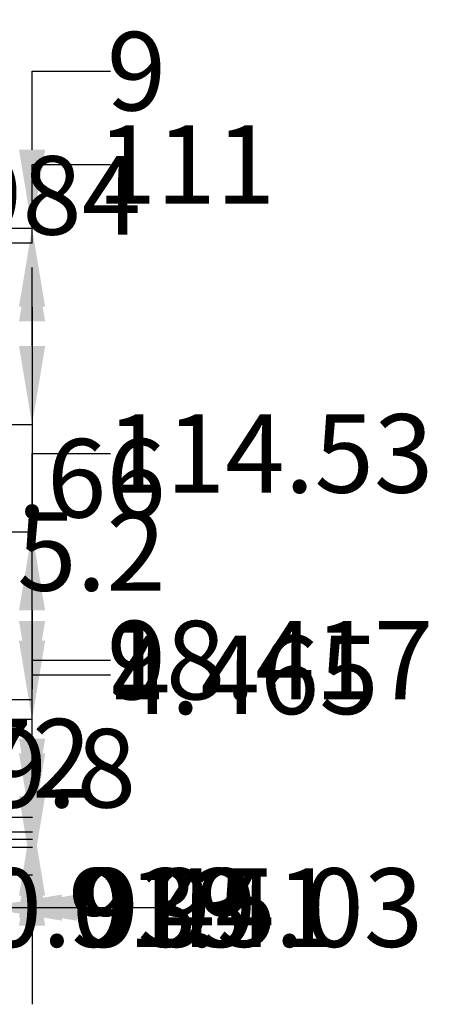
# Model space of a CAD drawing. Units: inches. Extents: x 131 to 858, y -65 to 554.
# Tile 4 of 4: x 605 to 858, y -48 to 554. Entities that reach past the tile are written whole.
import ezdxf

# ---------------------------------------------------------------- set-up
doc = ezdxf.new("R2010")
doc.units = ezdxf.units.IN
doc.header["$MEASUREMENT"] = 0
doc.layers.add('A-ANNO-DIMS', color=2, linetype='Continuous', lineweight=18)
doc.styles.get("Standard").update_dxf_attribs({"font": 'arial.ttf'})
doc.dimstyles.get("Standard").update_dxf_attribs({"dimtxt": 48, "dimasz": 48, "dimexe": 0.18, "dimexo": 0.0625, "dimgap": 0.09, "dimtad": 0, "dimtih": 1, "dimtoh": 1, "dimdec": 0, "dimrnd": 72, "dimzin": 0, "dimdsep": 46, "dimlunit": 3, "dimtxsty": 'Standard', "dimcen": 0.09, "dimadec": 0, "dimazin": 0, "dimtfac": 1, "dimtdec": 0, "dimtofl": 0, "dimtmove": 0, "dimatfit": 3, "dimfxl": 1, "dimtolj": 1, "dimtzin": 0, "dimarcsym": 0})

# ---------------------------------------------------------------- blocks, each defined once
blk = doc.blocks.new('*D5')
at = {"layer": 'A-ANNO-DIMS', "color": 0, "lineweight": -2, "transparency": 16777216}
for p, q in [((325.03, 446.65), (277.03, 446.65)), ((373.03, 426.61), (373.03, 446.83)), ((386.01, 421.76), (386.01, 446.83)), ((434.01, 446.65), (482.01, 446.65))]:
    blk.add_line(p, q, dxfattribs=at)
at = {"layer": 'A-ANNO-DIMS', "color": 0, "transparency": 16777216}
for points in [[(325.03, 454.65), (325.03, 438.65), (373.03, 446.65)], [(434.01, 454.65), (434.01, 438.65), (386.01, 446.65)]]:
    blk.add_solid(points, dxfattribs=at)
at = {"layer": 'Defpoints', "color": 0, "transparency": 16777216}
for p in [(386.01, 446.65), (373.03, 426.55), (386.01, 421.7)]:
    blk.add_point(p, dxfattribs=at)
at = {"layer": 'A-ANNO-DIMS', "color": 0, "transparency": 16777216, "insert": (579.38, 446.65), "char_height": 48, "attachment_point": 5}
blk.add_mtext('\\A1;12.984', dxfattribs=at)
blk = doc.blocks.new('*D11')
at = {"layer": 'A-ANNO-DIMS', "color": 0, "lineweight": -2, "transparency": 16777216}
for p, q in [((395.014446, 31.273524), (395.014446, 11.056024)), ((539.014446, 31.273524), (539.014446, 11.056024)), ((347.014446, 11.236024), (299.014446, 11.236024)), ((587.014446, 11.236024), (635.014446, 11.236024))]:
    blk.add_line(p, q, dxfattribs=at)
at = {"layer": 'A-ANNO-DIMS', "color": 0, "transparency": 16777216}
for points in [[(347.014446, 19.236024), (347.014446, 3.236024), (395.014446, 11.236024)], [(587.014446, 19.236024), (587.014446, 3.236024), (539.014446, 11.236024)]]:
    blk.add_solid(points, dxfattribs=at)
at = {"layer": 'Defpoints', "color": 0, "transparency": 16777216}
for p in [(395.014446, 31.336024), (539.014446, 31.336024), (539.014446, 11.236024)]:
    blk.add_point(p, dxfattribs=at)
at = {"layer": 'A-ANNO-DIMS', "color": 0, "transparency": 16777216, "insert": (467.014446, 11.236024), "char_height": 48, "attachment_point": 5}
blk.add_mtext('\\A1;144', dxfattribs=at)
blk = doc.blocks.new('*D12')
at = {"layer": 'A-ANNO-DIMS', "color": 0, "lineweight": -2, "transparency": 16777216}
for p, q in [((539.01, 31.27), (539.01, 11.06)), ((548.01, 31.27), (548.01, 11.06)), ((491.01, 11.24), (443.01, 11.24)), ((596.01, 11.24), (644.01, 11.24))]:
    blk.add_line(p, q, dxfattribs=at)
at = {"layer": 'A-ANNO-DIMS', "color": 0, "transparency": 16777216}
for points in [[(491.01, 19.24), (491.01, 3.24), (539.01, 11.24)], [(596.01, 19.24), (596.01, 3.24), (548.01, 11.24)]]:
    blk.add_solid(points, dxfattribs=at)
at = {"layer": 'Defpoints', "color": 0, "transparency": 16777216}
for p in [(539.01, 31.34), (548.01, 31.34), (548.01, 11.24)]:
    blk.add_point(p, dxfattribs=at)
at = {"layer": 'A-ANNO-DIMS', "color": 0, "transparency": 16777216, "insert": (659.89, 11.24), "char_height": 48, "attachment_point": 5}
blk.add_mtext('\\A1;9', dxfattribs=at)
blk = doc.blocks.new('*D13')
at = {"layer": 'A-ANNO-DIMS', "color": 0, "lineweight": -2, "transparency": 16777216}
for p, q in [((592.04, 126.29), (592.04, 11.06)), ((548.01, 31.27), (548.01, 11.06)), ((500.01, 11.24), (452.01, 11.24)), ((640.04, 11.24), (688.04, 11.24))]:
    blk.add_line(p, q, dxfattribs=at)
at = {"layer": 'A-ANNO-DIMS', "color": 0, "transparency": 16777216}
for points in [[(500.01, 19.24), (500.01, 3.24), (548.01, 11.24)], [(640.04, 19.24), (640.04, 3.24), (592.04, 11.24)]]:
    blk.add_solid(points, dxfattribs=at)
at = {"layer": 'Defpoints', "color": 0, "transparency": 16777216}
for p in [(592.04, 126.36), (548.01, 31.34), (592.04, 11.24)]:
    blk.add_point(p, dxfattribs=at)
at = {"layer": 'A-ANNO-DIMS', "color": 0, "transparency": 16777216, "insert": (770.09, 11.24), "char_height": 48, "attachment_point": 5}
blk.add_mtext('\\A1;44.03', dxfattribs=at)
blk = doc.blocks.new('*D14')
at = {"layer": 'A-ANNO-DIMS', "color": 0, "lineweight": -2, "transparency": 16777216}
for p, q in [((592.11, 426.55), (612.82, 426.55)), ((612.64, 378.55), (612.64, 253.56)), ((612.64, 79.34), (612.64, 204.33)), ((233.08, 31.34), (612.82, 31.34))]:
    blk.add_line(p, q, dxfattribs=at)
at = {"layer": 'A-ANNO-DIMS', "color": 0, "transparency": 16777216}
for points in [[(604.64, 378.55), (620.64, 378.55), (612.64, 426.55)], [(604.64, 79.34), (620.64, 79.34), (612.64, 31.34)]]:
    blk.add_solid(points, dxfattribs=at)
at = {"layer": 'Defpoints', "color": 0, "transparency": 16777216}
for p in [(592.04, 426.55), (612.64, 426.55), (233.01, 31.34)]:
    blk.add_point(p, dxfattribs=at)
at = {"layer": 'A-ANNO-DIMS', "color": 0, "transparency": 16777216, "insert": (612.64, 228.94), "char_height": 48, "attachment_point": 5}
blk.add_mtext('\\A1;395.2', dxfattribs=at)
blk = doc.blocks.new('*D19')
at = {"layer": 'A-ANNO-DIMS', "color": 0, "lineweight": -2, "transparency": 16777216}
for p, q in [((612.64, 105.55), (612.64, 153.55)), ((612.64, 153.55), (660.64, 153.55)), ((242.08, 57.55), (612.82, 57.55)), ((242.08, 53.09), (612.82, 53.09)), ((612.64, 5.09), (612.64, -42.91))]:
    blk.add_line(p, q, dxfattribs=at)
at = {"layer": 'A-ANNO-DIMS', "color": 0, "transparency": 16777216}
for points in [[(604.64, 105.55), (620.64, 105.55), (612.64, 57.55)], [(604.64, 5.09), (620.64, 5.09), (612.64, 53.09)]]:
    blk.add_solid(points, dxfattribs=at)
at = {"layer": 'Defpoints', "color": 0, "transparency": 16777216}
for p in [(242.01, 57.55), (612.64, 57.55), (242.01, 53.09)]:
    blk.add_point(p, dxfattribs=at)
at = {"layer": 'A-ANNO-DIMS', "color": 0, "transparency": 16777216, "insert": (742.86, 153.55), "char_height": 48, "attachment_point": 5}
blk.add_mtext('\\A1;4.465', dxfattribs=at)
blk = doc.blocks.new('*D20')
at = {"layer": 'A-ANNO-DIMS', "color": 0, "lineweight": -2, "transparency": 16777216}
for p, q in [((612.64, 114.55), (612.64, 162.55)), ((612.64, 162.55), (660.64, 162.55)), ((242.08, 66.55), (612.82, 66.55)), ((242.08, 57.55), (612.82, 57.55)), ((612.64, 9.55), (612.64, -38.45))]:
    blk.add_line(p, q, dxfattribs=at)
at = {"layer": 'A-ANNO-DIMS', "color": 0, "transparency": 16777216}
for points in [[(604.64, 114.55), (620.64, 114.55), (612.64, 66.55)], [(604.64, 9.55), (620.64, 9.55), (612.64, 57.55)]]:
    blk.add_solid(points, dxfattribs=at)
at = {"layer": 'Defpoints', "color": 0, "transparency": 16777216}
for p in [(242.01, 66.55), (612.64, 66.55), (242.01, 57.55)]:
    blk.add_point(p, dxfattribs=at)
at = {"layer": 'A-ANNO-DIMS', "color": 0, "transparency": 16777216, "insert": (676.51, 162.55), "char_height": 48, "attachment_point": 5}
blk.add_mtext('\\A1;9', dxfattribs=at)
blk = doc.blocks.new('*D22')
at = {"layer": 'A-ANNO-DIMS', "color": 0, "lineweight": -2, "transparency": 16777216}
for p, q in [((612.64, 114.55), (612.64, 162.55)), ((612.64, 162.55), (660.64, 162.55)), ((395.08, 66.55), (612.82, 66.55)), ((395.08, 48.13), (612.82, 48.13)), ((612.64, 0.13), (612.64, -47.87))]:
    blk.add_line(p, q, dxfattribs=at)
at = {"layer": 'A-ANNO-DIMS', "color": 0, "transparency": 16777216}
for points in [[(604.64, 114.55), (620.64, 114.55), (612.64, 66.55)], [(604.64, 0.13), (620.64, 0.13), (612.64, 48.13)]]:
    blk.add_solid(points, dxfattribs=at)
at = {"layer": 'Defpoints', "color": 0, "transparency": 16777216}
for p in [(395.01, 66.55), (612.64, 66.55), (395.01, 48.13)]:
    blk.add_point(p, dxfattribs=at)
at = {"layer": 'A-ANNO-DIMS', "color": 0, "transparency": 16777216, "insert": (758.11, 162.55), "char_height": 48, "attachment_point": 5}
blk.add_mtext('\\A1;18.417', dxfattribs=at)
blk = doc.blocks.new('*D30')
at = {"layer": 'A-ANNO-DIMS', "color": 0, "lineweight": -2, "transparency": 16777216}
for p, q in [((612.64, 417.55), (612.64, 465.55)), ((612.64, 465.55), (660.64, 465.55)), ((592.11, 417.55), (612.82, 417.55)), ((612.64, 354.55), (612.64, 369.55)), ((443.08, 306.55), (612.82, 306.55))]:
    blk.add_line(p, q, dxfattribs=at)
at = {"layer": 'A-ANNO-DIMS', "color": 0, "transparency": 16777216}
for points in [[(604.64, 369.55), (620.64, 369.55), (612.64, 417.55)], [(604.64, 354.55), (620.64, 354.55), (612.64, 306.55)]]:
    blk.add_solid(points, dxfattribs=at)
at = {"layer": 'Defpoints', "color": 0, "transparency": 16777216}
for p in [(592.04, 417.55), (612.64, 417.55), (443.01, 306.55)]:
    blk.add_point(p, dxfattribs=at)
at = {"layer": 'A-ANNO-DIMS', "color": 0, "transparency": 16777216, "insert": (706.86, 465.55), "char_height": 48, "attachment_point": 5}
blk.add_mtext('\\A1;111', dxfattribs=at)
blk = doc.blocks.new('*D31')
at = {"layer": 'A-ANNO-DIMS', "color": 0, "lineweight": -2, "transparency": 16777216}
for p, q in [((612.64, 474.55), (612.64, 522.55)), ((612.64, 522.55), (660.64, 522.55)), ((592.11, 426.55), (612.82, 426.55)), ((592.11, 417.55), (612.82, 417.55)), ((612.64, 369.55), (612.64, 321.55))]:
    blk.add_line(p, q, dxfattribs=at)
at = {"layer": 'A-ANNO-DIMS', "color": 0, "transparency": 16777216}
for points in [[(604.64, 474.55), (620.64, 474.55), (612.64, 426.55)], [(604.64, 369.55), (620.64, 369.55), (612.64, 417.55)]]:
    blk.add_solid(points, dxfattribs=at)
at = {"layer": 'Defpoints', "color": 0, "transparency": 16777216}
for p in [(592.04, 426.55), (612.64, 426.55), (592.04, 417.55)]:
    blk.add_point(p, dxfattribs=at)
at = {"layer": 'A-ANNO-DIMS', "color": 0, "transparency": 16777216, "insert": (676.51, 522.55), "char_height": 48, "attachment_point": 5}
blk.add_mtext('\\A1;9', dxfattribs=at)
blk = doc.blocks.new('*D33')
at = {"layer": 'A-ANNO-DIMS', "color": 0, "lineweight": -2, "transparency": 16777216}
for p, q in [((612.639956, 186.551418), (612.639956, 234.551418)), ((431.076946, 138.551418), (612.819956, 138.551418)), ((431.076946, 66.551418), (612.819956, 66.551418)), ((612.639956, 18.551418), (612.639956, -29.448582))]:
    blk.add_line(p, q, dxfattribs=at)
at = {"layer": 'A-ANNO-DIMS', "color": 0, "transparency": 16777216}
for points in [[(604.639956, 186.551418), (620.639956, 186.551418), (612.639956, 138.551418)], [(604.639956, 18.551418), (620.639956, 18.551418), (612.639956, 66.551418)]]:
    blk.add_solid(points, dxfattribs=at)
at = {"layer": 'Defpoints', "color": 0, "transparency": 16777216}
for p in [(431.014446, 138.551418), (612.639956, 138.551418), (431.014446, 66.551418)]:
    blk.add_point(p, dxfattribs=at)
at = {"layer": 'A-ANNO-DIMS', "color": 0, "transparency": 16777216, "insert": (612.639956, 102.551418), "char_height": 48, "attachment_point": 5}
blk.add_mtext('\\A1;72', dxfattribs=at)
blk = doc.blocks.new('*D36')
at = {"layer": 'A-ANNO-DIMS', "color": 0, "lineweight": -2, "transparency": 16777216}
for p, q in [((452.53, 73.54), (452.53, 11.06)), ((442.52, 66.49), (442.52, 11.06)), ((394.52, 11.24), (346.52, 11.24)), ((500.53, 11.24), (548.53, 11.24))]:
    blk.add_line(p, q, dxfattribs=at)
at = {"layer": 'A-ANNO-DIMS', "color": 0, "transparency": 16777216}
for points in [[(394.52, 19.24), (394.52, 3.24), (442.52, 11.24)], [(500.53, 19.24), (500.53, 3.24), (452.53, 11.24)]]:
    blk.add_solid(points, dxfattribs=at)
at = {"layer": 'Defpoints', "color": 0, "transparency": 16777216}
for p in [(452.53, 73.6), (442.52, 66.55), (452.53, 11.24)]:
    blk.add_point(p, dxfattribs=at)
at = {"layer": 'A-ANNO-DIMS', "color": 0, "transparency": 16777216, "insert": (646, 11.24), "char_height": 48, "attachment_point": 5}
blk.add_mtext('\\A1;10.013', dxfattribs=at)
blk = doc.blocks.new('*D37')
at = {"layer": 'A-ANNO-DIMS', "color": 0, "lineweight": -2, "transparency": 16777216}
for p, q in [((544.04, 126.29), (544.04, 11.06)), ((452.53, 73.54), (452.53, 11.06)), ((404.53, 11.24), (356.53, 11.24)), ((592.04, 11.24), (640.04, 11.24))]:
    blk.add_line(p, q, dxfattribs=at)
at = {"layer": 'A-ANNO-DIMS', "color": 0, "transparency": 16777216}
for points in [[(404.53, 19.24), (404.53, 3.24), (452.53, 11.24)], [(592.04, 19.24), (592.04, 3.24), (544.04, 11.24)]]:
    blk.add_solid(points, dxfattribs=at)
at = {"layer": 'Defpoints', "color": 0, "transparency": 16777216}
for p in [(544.04, 126.36), (452.53, 73.6), (544.04, 11.24)]:
    blk.add_point(p, dxfattribs=at)
at = {"layer": 'A-ANNO-DIMS', "color": 0, "transparency": 16777216, "insert": (716.49, 11.24), "char_height": 48, "attachment_point": 5}
blk.add_mtext('\\A1;91.51', dxfattribs=at)
blk = doc.blocks.new('*D38')
at = {"layer": 'A-ANNO-DIMS', "color": 0, "lineweight": -2, "transparency": 16777216}
for p, q in [((544.04, 126.29), (544.04, 11.06)), ((583.04, 126.29), (583.04, 11.06)), ((496.04, 11.24), (448.04, 11.24)), ((631.04, 11.24), (679.04, 11.24))]:
    blk.add_line(p, q, dxfattribs=at)
at = {"layer": 'A-ANNO-DIMS', "color": 0, "transparency": 16777216}
for points in [[(496.04, 19.24), (496.04, 3.24), (544.04, 11.24)], [(631.04, 19.24), (631.04, 3.24), (583.04, 11.24)]]:
    blk.add_solid(points, dxfattribs=at)
at = {"layer": 'Defpoints', "color": 0, "transparency": 16777216}
for p in [(544.04, 126.36), (583.04, 126.36), (583.04, 11.24)]:
    blk.add_point(p, dxfattribs=at)
at = {"layer": 'A-ANNO-DIMS', "color": 0, "transparency": 16777216, "insert": (713.55, 11.24), "char_height": 48, "attachment_point": 5}
blk.add_mtext('\\A1;39', dxfattribs=at)
blk = doc.blocks.new('*D39')
at = {"layer": 'A-ANNO-DIMS', "color": 0, "lineweight": -2, "transparency": 16777216}
for p, q in [((583.04, 126.29), (583.04, 11.06)), ((592.04, 126.29), (592.04, 11.06)), ((535.04, 11.24), (487.04, 11.24)), ((640.04, 11.24), (688.04, 11.24))]:
    blk.add_line(p, q, dxfattribs=at)
at = {"layer": 'A-ANNO-DIMS', "color": 0, "transparency": 16777216}
for points in [[(535.04, 19.24), (535.04, 3.24), (583.04, 11.24)], [(640.04, 19.24), (640.04, 3.24), (592.04, 11.24)]]:
    blk.add_solid(points, dxfattribs=at)
at = {"layer": 'Defpoints', "color": 0, "transparency": 16777216}
for p in [(583.04, 126.36), (592.04, 126.36), (592.04, 11.24)]:
    blk.add_point(p, dxfattribs=at)
at = {"layer": 'A-ANNO-DIMS', "color": 0, "transparency": 16777216, "insert": (703.92, 11.24), "char_height": 48, "attachment_point": 5}
blk.add_mtext('\\A1;9', dxfattribs=at)
blk = doc.blocks.new('*D41')
at = {"layer": 'A-ANNO-DIMS', "color": 0, "lineweight": -2, "transparency": 16777216}
for p, q in [((612.64, 174.36), (612.64, 222.36)), ((592.11, 126.36), (612.82, 126.36)), ((548.08, 66.55), (612.82, 66.55)), ((612.64, 18.55), (612.64, -29.45))]:
    blk.add_line(p, q, dxfattribs=at)
at = {"layer": 'A-ANNO-DIMS', "color": 0, "transparency": 16777216}
for points in [[(604.64, 174.36), (620.64, 174.36), (612.64, 126.36)], [(604.64, 18.55), (620.64, 18.55), (612.64, 66.55)]]:
    blk.add_solid(points, dxfattribs=at)
at = {"layer": 'Defpoints', "color": 0, "transparency": 16777216}
for p in [(592.04, 126.36), (612.64, 126.36), (548.01, 66.55)]:
    blk.add_point(p, dxfattribs=at)
at = {"layer": 'A-ANNO-DIMS', "color": 0, "transparency": 16777216, "insert": (612.64, 96.45), "char_height": 48, "attachment_point": 5}
blk.add_mtext('\\A1;59.8', dxfattribs=at)
blk = doc.blocks.new('*D42')
at = {"layer": 'A-ANNO-DIMS', "color": 0, "lineweight": -2, "transparency": 16777216}
for p, q in [((612.64, 240.89), (612.64, 288.89)), ((612.64, 288.89), (660.64, 288.89)), ((592.6, 240.89), (612.82, 240.89)), ((612.64, 174.36), (612.64, 192.89)), ((592.11, 126.36), (612.82, 126.36))]:
    blk.add_line(p, q, dxfattribs=at)
at = {"layer": 'A-ANNO-DIMS', "color": 0, "transparency": 16777216}
for points in [[(604.64, 192.89), (620.64, 192.89), (612.64, 240.89)], [(604.64, 174.36), (620.64, 174.36), (612.64, 126.36)]]:
    blk.add_solid(points, dxfattribs=at)
at = {"layer": 'Defpoints', "color": 0, "transparency": 16777216}
for p in [(592.54, 240.89), (612.64, 240.89), (592.04, 126.36)]:
    blk.add_point(p, dxfattribs=at)
at = {"layer": 'A-ANNO-DIMS', "color": 0, "transparency": 16777216, "insert": (758.11, 288.89), "char_height": 48, "attachment_point": 5}
blk.add_mtext('\\A1;114.53', dxfattribs=at)
blk = doc.blocks.new('*D43')
at = {"layer": 'A-ANNO-DIMS', "color": 0, "lineweight": -2, "transparency": 16777216}
for p, q in [((612.639956, 354.551418), (612.639956, 402.551418)), ((443.076946, 306.551418), (612.819956, 306.551418)), ((592.602456, 240.886672), (612.819956, 240.886672)), ((612.639956, 192.886672), (612.639956, 144.886672))]:
    blk.add_line(p, q, dxfattribs=at)
at = {"layer": 'A-ANNO-DIMS', "color": 0, "transparency": 16777216}
for points in [[(604.639956, 354.551418), (620.639956, 354.551418), (612.639956, 306.551418)], [(604.639956, 192.886672), (620.639956, 192.886672), (612.639956, 240.886672)]]:
    blk.add_solid(points, dxfattribs=at)
at = {"layer": 'Defpoints', "color": 0, "transparency": 16777216}
for p in [(443.014446, 306.551418), (612.639956, 306.551418), (592.539956, 240.886672)]:
    blk.add_point(p, dxfattribs=at)
at = {"layer": 'A-ANNO-DIMS', "color": 0, "transparency": 16777216, "insert": (612.639956, 273.719045), "char_height": 48, "attachment_point": 5}
blk.add_mtext('\\A1;65.66', dxfattribs=at)

msp = doc.modelspace()

# ---------------------------------------------------------------- dimensions: what is measured, and where the dimension line sits
at = {"layer": 'A-ANNO-DIMS'}
for base, p1, p2, override, picture, middle in [((612.64, 426.5514), (592.0434, 417.5514), (592.0434, 426.5514), {"dimdec": 0, "dimlfac": 1, "dimrnd": 0, "dimzin": 0, "dimdsep": 46, "dimlunit": 2}, '*D31', (676.5117, 522.5514)), ((612.64, 417.5514), (443.0144, 306.5514), (592.0434, 417.5514), {"dimdec": 0, "dimlfac": 1, "dimrnd": 0, "dimzin": 0, "dimdsep": 46, "dimlunit": 2}, '*D30', (706.8637, 465.5514)), ((612.64, 426.5514), (233.0144, 31.336), (592.0434, 426.5514), {"dimdec": 1, "dimlfac": 1, "dimrnd": 0, "dimzin": 0, "dimdsep": 46, "dimlunit": 2}, '*D14', (612.64, 228.9437)), ((612.64, 306.5514), (592.54, 240.8867), (443.0144, 306.5514), {"dimdec": 2, "dimlfac": 1, "dimrnd": 0, "dimzin": 0, "dimdsep": 46, "dimlunit": 2}, '*D43', (612.64, 273.719)), ((612.64, 240.8867), (592.0434, 126.3568), (592.54, 240.8867), {"dimdec": 2, "dimlfac": 1, "dimrnd": 0, "dimzin": 0, "dimdsep": 46, "dimlunit": 2}, '*D42', (758.1051, 288.8867)), ((612.64, 138.5514), (431.0144, 66.5514), (431.0144, 138.5514), {"dimdec": 0, "dimlfac": 1, "dimrnd": 0, "dimzin": 0, "dimdsep": 46, "dimlunit": 2}, '*D33', (612.64, 102.5514)), ((612.64, 126.3568), (548.0144, 66.5514), (592.0434, 126.3568), {"dimdec": 1, "dimlfac": 1, "dimrnd": 0, "dimzin": 0, "dimdsep": 46, "dimlunit": 2}, '*D41', (612.64, 96.4541)), ((612.64, 66.5514), (242.0144, 57.5514), (242.0144, 66.5514), {"dimdec": 0, "dimlfac": 1, "dimrnd": 0, "dimzin": 0, "dimdsep": 46, "dimlunit": 2}, '*D20', (676.5117, 162.5514)), ((612.64, 66.5514), (395.0144, 48.1342), (395.0144, 66.5514), {"dimdec": 3, "dimlfac": 1, "dimrnd": 0, "dimzin": 0, "dimdsep": 46, "dimlunit": 2}, '*D22', (758.1051, 162.5514)), ((612.64, 57.5514), (242.0144, 53.0868), (242.0144, 57.5514), {"dimdec": 3, "dimlfac": 1, "dimrnd": 0, "dimzin": 0, "dimdsep": 46, "dimlunit": 2}, '*D19', (742.8637, 153.5514))]:
    dim = msp.add_linear_dim(base=base, p1=p1, p2=p2, angle=90, dimstyle='Standard', override=override, dxfattribs=at)
    dim.commit()
    dim.dimension.update_dxf_attribs({"geometry": picture, "text_midpoint": middle})
for base, p1, p2, override, picture, middle in [((386.0144, 446.6514), (373.0302, 426.5514), (386.0144, 421.6997), {"dimdec": 3, "dimlfac": 1, "dimrnd": 0, "dimzin": 0, "dimdsep": 46, "dimlunit": 2}, '*D5', (579.3814, 446.6514)), ((544.0434, 11.236), (452.5306, 73.6016), (544.0434, 126.3568), {"dimdec": 2, "dimlfac": 1, "dimrnd": 0, "dimzin": 0, "dimdsep": 46, "dimlunit": 2}, '*D37', (716.4881, 11.236)), ((583.0434, 11.236), (544.0434, 126.3568), (583.0434, 126.3568), {"dimdec": 0, "dimlfac": 1, "dimrnd": 0, "dimzin": 0, "dimdsep": 46, "dimlunit": 2}, '*D38', (713.5454, 11.236)), ((592.0434, 11.236), (548.0144, 31.336), (592.0434, 126.3568), {"dimdec": 2, "dimlfac": 1, "dimrnd": 0, "dimzin": 0, "dimdsep": 46, "dimlunit": 2}, '*D13', (770.0871, 11.236)), ((592.0434, 11.236), (583.0434, 126.3568), (592.0434, 126.3568), {"dimdec": 0, "dimlfac": 1, "dimrnd": 0, "dimzin": 0, "dimdsep": 46, "dimlunit": 2}, '*D39', (703.9152, 11.236)), ((452.5306, 11.236), (442.5179, 66.5514), (452.5306, 73.6016), {"dimdec": 3, "dimlfac": 1, "dimrnd": 0, "dimzin": 0, "dimdsep": 46, "dimlunit": 2}, '*D36', (645.9958, 11.236)), ((539.0144, 11.236), (395.0144, 31.336), (539.0144, 31.336), {"dimdec": 0, "dimlfac": 1, "dimrnd": 0, "dimzin": 0, "dimdsep": 46, "dimlunit": 2}, '*D11', (467.0144, 11.236)), ((548.0144, 11.236), (539.0144, 31.336), (548.0144, 31.336), {"dimdec": 0, "dimlfac": 1, "dimrnd": 0, "dimzin": 0, "dimdsep": 46, "dimlunit": 2}, '*D12', (659.8862, 11.236))]:
    dim = msp.add_linear_dim(base=base, p1=p1, p2=p2, dimstyle='Standard', override=override, dxfattribs=at)
    dim.commit()
    dim.dimension.update_dxf_attribs({"geometry": picture, "text_midpoint": middle})

doc.saveas('drawing.dxf')
